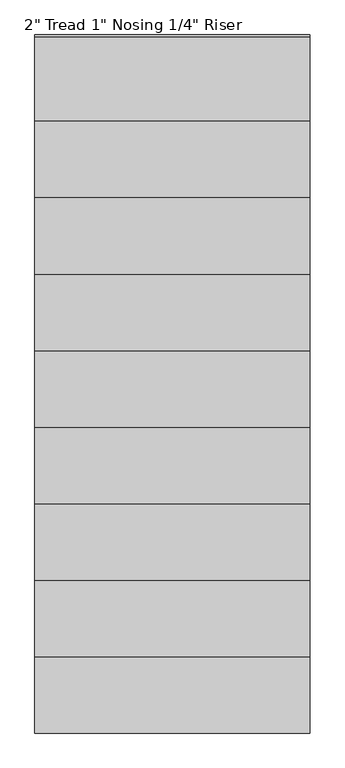
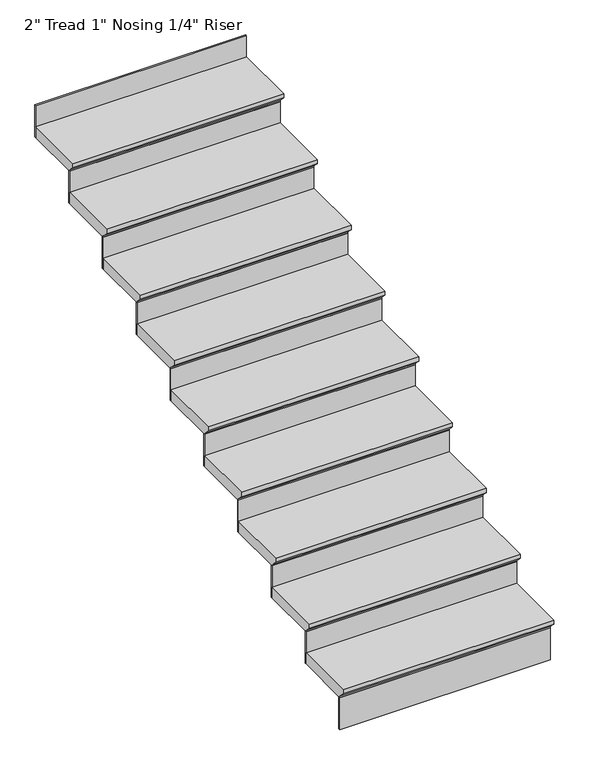
"""IFC4 building model written with IfcOpenShell, lengths in millimetres: stair flight geometry."""

from ifc_helpers import new_model, si_unit, frame, origin, place, context, project, spatial, polyline, outline, extrude, source, transform, mapped, element, save


def stair_flight_dd50f657(model_context):
    return source(origin(), model_context, "Body", "SweptSolid", [
        extrude(outline(polyline([(-6527.0593836, 14371.1107431), (-6247.6593836, 14371.1107431), (-6247.6593836, 14320.3107431), (-6501.6593836, 14320.3107431), (-6501.6593836, 14326.6607431), (-6527.0593836, 14352.0607431), (-6527.0593836, 14371.1107431)])), frame((-5280.3137331, 0.0, 0.0), z_axis=(1.0, 0.0, 0.0), x_axis=(0.0, 1.0, 0.0)), (0.0, 0.0, 1.0), 914.4),
        extrude(outline(polyline([(-4365.9137331, -6495.3093836), (-4365.9137331, -6501.6593836), (-5280.3137331, -6501.6593836), (-5280.3137331, -6495.3093836), (-4365.9137331, -6495.3093836)])), frame((0.0, 0.0, 14172.4618174), z_axis=(0.0, 0.0, 1.0), x_axis=(1.0, 0.0, 0.0)), (0.0, 0.0, 1.0), 147.8489257),
        extrude(outline(polyline([(-4365.9137331, -6241.3093836), (-4365.9137331, -6247.6593836), (-5280.3137331, -6247.6593836), (-5280.3137331, -6241.3093836), (-4365.9137331, -6241.3093836)])), frame((0.0, 0.0, 14320.3107431), z_axis=(0.0, 0.0, 1.0), x_axis=(1.0, 0.0, 0.0)), (0.0, 0.0, 1.0), 147.8489257),
        extrude(outline(polyline([(-6273.0593836, 14518.9596688), (-5993.6593836, 14518.9596688), (-5993.6593836, 14468.1596688), (-6247.6593836, 14468.1596688), (-6247.6593836, 14474.5096688), (-6273.0593836, 14499.9096688), (-6273.0593836, 14518.9596688)])), frame((-5280.3137331, 0.0, 0.0), z_axis=(1.0, 0.0, 0.0), x_axis=(0.0, 1.0, 0.0)), (0.0, 0.0, 1.0), 914.4),
        extrude(outline(polyline([(-4365.9137331, -5987.3093836), (-4365.9137331, -5993.6593836), (-5280.3137331, -5993.6593836), (-5280.3137331, -5987.3093836), (-4365.9137331, -5987.3093836)])), frame((0.0, 0.0, 14468.1596688), z_axis=(0.0, 0.0, 1.0), x_axis=(1.0, 0.0, 0.0)), (0.0, 0.0, 1.0), 147.8489257),
        extrude(outline(polyline([(-6019.0593836, 14666.8085944), (-5739.6593836, 14666.8085944), (-5739.6593836, 14616.0085944), (-5993.6593836, 14616.0085944), (-5993.6593836, 14622.3585944), (-6019.0593836, 14647.7585944), (-6019.0593836, 14666.8085944)])), frame((-5280.3137331, 0.0, 0.0), z_axis=(1.0, 0.0, 0.0), x_axis=(0.0, 1.0, 0.0)), (0.0, 0.0, 1.0), 914.4),
        extrude(outline(polyline([(-4365.9137331, -5733.3093836), (-4365.9137331, -5739.6593836), (-5280.3137331, -5739.6593836), (-5280.3137331, -5733.3093836), (-4365.9137331, -5733.3093836)])), frame((0.0, 0.0, 14616.0085944), z_axis=(0.0, 0.0, 1.0), x_axis=(1.0, 0.0, 0.0)), (0.0, 0.0, 1.0), 147.8489257),
        extrude(outline(polyline([(-5765.0593836, 14814.6575201), (-5485.6593836, 14814.6575201), (-5485.6593836, 14763.8575201), (-5739.6593836, 14763.8575201), (-5739.6593836, 14770.2075201), (-5765.0593836, 14795.6075201), (-5765.0593836, 14814.6575201)])), frame((-5280.3137331, 0.0, 0.0), z_axis=(1.0, 0.0, 0.0), x_axis=(0.0, 1.0, 0.0)), (0.0, 0.0, 1.0), 914.4),
        extrude(outline(polyline([(-4365.9137331, -5479.3093836), (-4365.9137331, -5485.6593836), (-5280.3137331, -5485.6593836), (-5280.3137331, -5479.3093836), (-4365.9137331, -5479.3093836)])), frame((0.0, 0.0, 14763.8575201), z_axis=(0.0, 0.0, 1.0), x_axis=(1.0, 0.0, 0.0)), (0.0, 0.0, 1.0), 147.8489257),
        extrude(outline(polyline([(-5511.0593836, 14962.5064458), (-5231.6593836, 14962.5064458), (-5231.6593836, 14911.7064458), (-5485.6593836, 14911.7064458), (-5485.6593836, 14918.0564458), (-5511.0593836, 14943.4564458), (-5511.0593836, 14962.5064458)])), frame((-5280.3137331, 0.0, 0.0), z_axis=(1.0, 0.0, 0.0), x_axis=(0.0, 1.0, 0.0)), (0.0, 0.0, 1.0), 914.4),
        extrude(outline(polyline([(-4365.9137331, -5225.3093836), (-4365.9137331, -5231.6593836), (-5280.3137331, -5231.6593836), (-5280.3137331, -5225.3093836), (-4365.9137331, -5225.3093836)])), frame((0.0, 0.0, 14911.7064458), z_axis=(0.0, 0.0, 1.0), x_axis=(1.0, 0.0, 0.0)), (0.0, 0.0, 1.0), 147.8489257),
        extrude(outline(polyline([(-5257.0593836, 15110.3553715), (-4977.6593836, 15110.3553715), (-4977.6593836, 15059.5553715), (-5231.6593836, 15059.5553715), (-5231.6593836, 15065.9053715), (-5257.0593836, 15091.3053715), (-5257.0593836, 15110.3553715)])), frame((-5280.3137331, 0.0, 0.0), z_axis=(1.0, 0.0, 0.0), x_axis=(0.0, 1.0, 0.0)), (0.0, 0.0, 1.0), 914.4),
        extrude(outline(polyline([(-4365.9137331, -4971.3093836), (-4365.9137331, -4977.6593836), (-5280.3137331, -4977.6593836), (-5280.3137331, -4971.3093836), (-4365.9137331, -4971.3093836)])), frame((0.0, 0.0, 15059.5553715), z_axis=(0.0, 0.0, 1.0), x_axis=(1.0, 0.0, 0.0)), (0.0, 0.0, 1.0), 147.8489257),
        extrude(outline(polyline([(-5003.0593836, 15258.2042972), (-4723.6593836, 15258.2042972), (-4723.6593836, 15207.4042972), (-4977.6593836, 15207.4042972), (-4977.6593836, 15213.7542972), (-5003.0593836, 15239.1542972), (-5003.0593836, 15258.2042972)])), frame((-5280.3137331, 0.0, 0.0), z_axis=(1.0, 0.0, 0.0), x_axis=(0.0, 1.0, 0.0)), (0.0, 0.0, 1.0), 914.4),
        extrude(outline(polyline([(-4365.9137331, -4717.3093836), (-4365.9137331, -4723.6593836), (-5280.3137331, -4723.6593836), (-5280.3137331, -4717.3093836), (-4365.9137331, -4717.3093836)])), frame((0.0, 0.0, 15207.4042972), z_axis=(0.0, 0.0, 1.0), x_axis=(1.0, 0.0, 0.0)), (0.0, 0.0, 1.0), 147.8489257),
        extrude(outline(polyline([(-4749.0593836, 15406.0532229), (-4469.6593836, 15406.0532229), (-4469.6593836, 15355.2532229), (-4723.6593836, 15355.2532229), (-4723.6593836, 15361.6032229), (-4749.0593836, 15387.0032229), (-4749.0593836, 15406.0532229)])), frame((-5280.3137331, 0.0, 0.0), z_axis=(1.0, 0.0, 0.0), x_axis=(0.0, 1.0, 0.0)), (0.0, 0.0, 1.0), 914.4),
        extrude(outline(polyline([(-4365.9137331, -4463.3093836), (-4365.9137331, -4469.6593836), (-5280.3137331, -4469.6593836), (-5280.3137331, -4463.3093836), (-4365.9137331, -4463.3093836)])), frame((0.0, 0.0, 15355.2532229), z_axis=(0.0, 0.0, 1.0), x_axis=(1.0, 0.0, 0.0)), (0.0, 0.0, 1.0), 147.8489257),
        extrude(outline(polyline([(-4365.9137331, -4209.3093836), (-4365.9137331, -4215.6593836), (-5280.3137331, -4215.6593836), (-5280.3137331, -4209.3093836), (-4365.9137331, -4209.3093836)])), frame((0.0, 0.0, 15503.1021486), z_axis=(0.0, 0.0, 1.0), x_axis=(1.0, 0.0, 0.0)), (0.0, 0.0, 1.0), 147.8489257),
        extrude(outline(polyline([(-4495.0593836, 15553.9021486), (-4215.6593836, 15553.9021486), (-4215.6593836, 15503.1021486), (-4469.6593836, 15503.1021486), (-4469.6593836, 15509.4521486), (-4495.0593836, 15534.8521486), (-4495.0593836, 15553.9021486)])), frame((-5280.3137331, 0.0, 0.0), z_axis=(1.0, 0.0, 0.0), x_axis=(0.0, 1.0, 0.0)), (0.0, 0.0, 1.0), 914.4),
    ])


if __name__ == "__main__":
    model = new_model("IFC4")
    model_context = context("Model", 3, world=origin())
    ifc_project = project(units=[si_unit("LENGTHUNIT", "METRE", prefix="MILLI")], contexts=[model_context])
    site = spatial("IfcSite", under=ifc_project)
    building = spatial("IfcBuilding", under=site)
    placement = place(None, origin())
    stair_flight_shape = stair_flight_dd50f657(model_context)
    element("IfcStairFlight", 1, ObjectType="2\" Tread 1\" Nosing 1/4\" Riser", at=placement, inside=building, context=model_context, shape_type="MappedRepresentation", body=[
        mapped(stair_flight_shape, transform((0.0, 0.0, 0.0), x_axis=(1.0, 0.0, 0.0), y_axis=(0.0, 1.0, 0.0), z_axis=(0.0, 0.0, 1.0))),
    ])
    save(model, "model.ifc")
